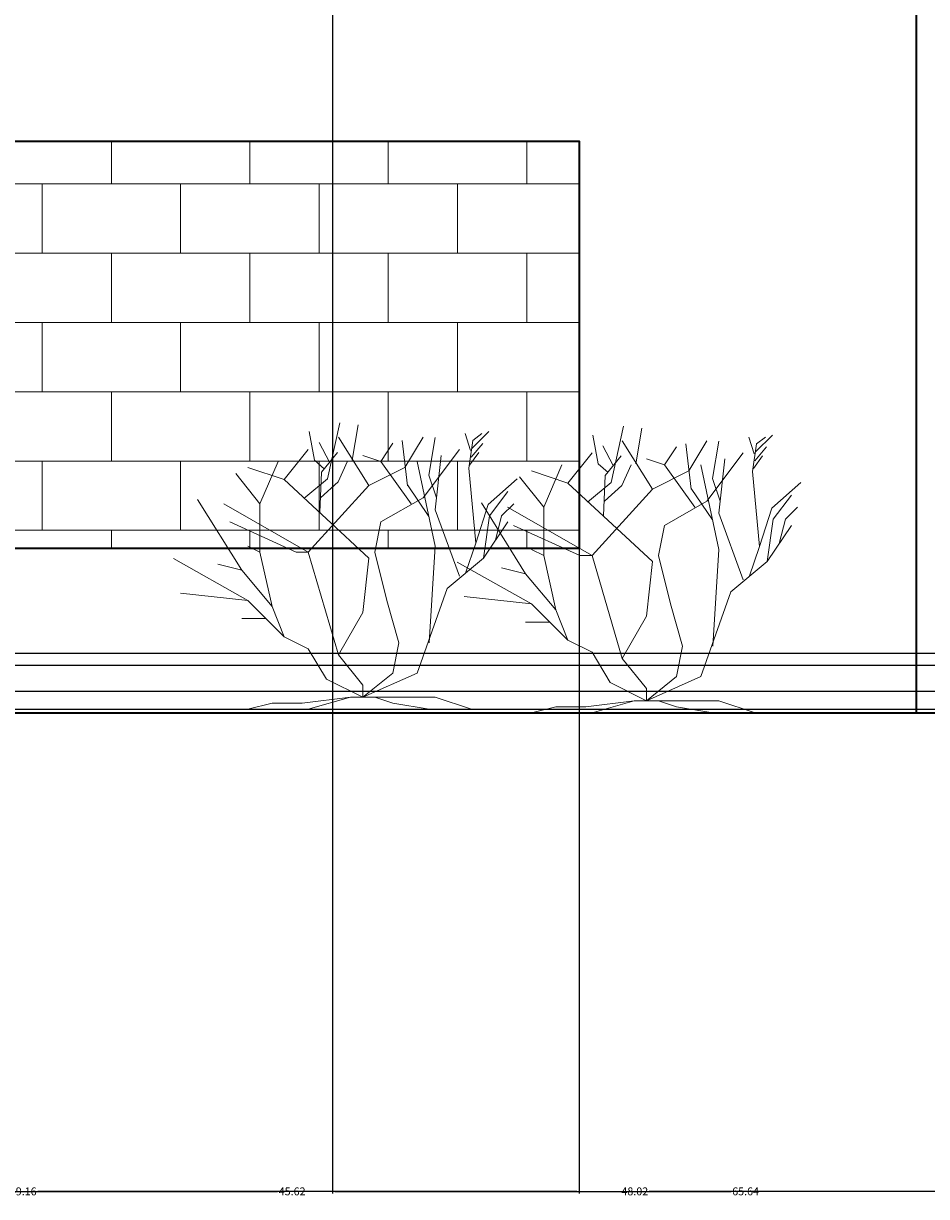
# Model space of a CAD drawing. Units: inches. Extents: x -13 to 809, y 112 to 656.
# Tile 8 of 55: x 186 to 257, y 112 to 205. Entities that reach past the tile are written whole.
import ezdxf

# ---------------------------------------------------------------- set-up
doc = ezdxf.new("R2010")
doc.units = ezdxf.units.IN
doc.header["$MEASUREMENT"] = 0
for name, color, linetype, lineweight in [('A-ANNO-DIMS', 2, 'Continuous', 18), ('A-ELEV', 7, 'Continuous', 35), ('A-ELEV-PATT', 8, 'Continuous', 13), ('L-PLNT', 3, 'Continuous', 18)]:
    doc.layers.add(name, color=color, linetype=linetype, lineweight=lineweight)
doc.styles.get("Standard").update_dxf_attribs({"font": 'arial.ttf'})
doc.dimstyles.get("Standard").update_dxf_attribs({"dimtxt": 0.625, "dimasz": 0.18, "dimexe": 0.18, "dimexo": 0.0625, "dimgap": 0.09, "dimtad": 0, "dimtih": 1, "dimtoh": 1, "dimdec": 4, "dimzin": 0, "dimdsep": 46, "dimlunit": 4, "dimtxsty": 'Standard', "dimcen": 0.09, "dimadec": 0, "dimazin": 0, "dimtfac": 1, "dimtdec": 4, "dimtofl": 0, "dimtmove": 0, "dimatfit": 3, "dimfxl": 1, "dimtolj": 1, "dimtzin": 0, "dimarcsym": 0})

# ---------------------------------------------------------------- blocks, each defined once
blk = doc.blocks.new('Shrub - elevation')
for p, q in [((-11.433, 18.289), (-10.457, 22.749)), ((-9.48, 19.775), (-8.992, 22.592)), ((-12.471, 19.775), (-12.898, 22.044)), ((-8.16, 17.76), (-10.56, 21.6)), ((-5.28, 19.2), (-3.84, 21.6)), ((-3.377, 18.602), (-2.888, 21.575)), ((-0.508, 21.888), (-0.081, 20.558)), ((0.041, 20.714), (1.384, 22.044)), ((0.102, 21.34), (0.835, 21.888)), ((-14.88, 18.24), (-12.96, 20.64)), ((-11.28, 19.619), (-12.104, 21.184)), ((-7.2, 19.68), (-6.24, 21.12)), ((-5.086, 17.741), (-5.513, 21.34)), ((-3.84, 16.8), (-0.96, 20.64)), ((-0.203, 19.149), (0.102, 21.34)), ((-0.02, 20.01), (0.896, 21.105)), ((-16.8, 16.32), (-15.36, 19.68)), ((-11.677, 19.071), (-12.471, 19.775)), ((-11.921, 18.836), (-10.64, 20.401)), ((-10.579, 18.054), (-9.846, 19.697)), ((-7.2, 19.68), (-8.64, 20.16)), ((-4.8, 16.32), (-7.2, 19.68)), ((-2.88, 12.96), (-4.32, 19.68)), ((-2.88, 15.84), (-2.4, 20.16)), ((-0.142, 19.384), (0.59, 20.401)), ((-16.8, 16.32), (-18.72, 18.72)), ((-14.88, 18.24), (-17.76, 19.2)), ((-12.043, 15.628), (-11.921, 18.836)), ((-8.16, 17.76), (-5.28, 19.2)), ((0.346, 13.203), (-0.203, 19.149)), ((-8.16, 12), (-14.88, 18.24)), ((-13.325, 16.724), (-11.433, 18.289)), ((-12.96, 12.48), (-8.16, 17.76)), ((-11.982, 16.802), (-10.579, 18.054)), ((-3.377, 15.315), (-5.086, 17.819)), ((-2.766, 16.802), (-3.377, 18.602)), ((1.323, 16.254), (3.642, 18.289)), ((-7.2, 14.88), (-3.84, 16.8)), ((1.44, 15.36), (2.88, 17.28)), ((-18.24, 11.04), (-21.755, 16.655)), ((-12.96, 12.48), (-19.68, 16.32)), ((-16.8, 12.48), (-16.8, 16.32)), ((-0.96, 10.56), (-2.88, 15.84)), ((0.346, 13.203), (1.323, 16.254)), ((2.4, 15.36), (3.36, 16.32)), ((0.96, 12), (1.44, 15.36)), ((1.92, 13.44), (2.4, 15.36)), ((-13.92, 12.48), (-19.2, 14.88)), ((-7.68, 12.48), (-7.2, 14.88)), ((0.96, 12), (2.88, 14.88)), ((-0.48, 10.8), (0.346, 13.203)), ((-16.8, 12.48), (-17.76, 12.96)), ((-15.84, 8.16), (-16.8, 12.48)), ((-12.96, 12.48), (-13.92, 12.48)), ((-10.56, 4.32), (-12.96, 12.48)), ((-6.72, 8.64), (-7.68, 12.48)), ((-3.36, 5.28), (-2.88, 12.96)), ((-17.76, 8.64), (-23.663, 11.961)), ((-18.24, 11.04), (-20.16, 11.52)), ((-8.64, 7.68), (-8.16, 12)), ((-1.92, 9.6), (0.96, 12)), ((-15.84, 8.16), (-18.24, 11.04)), ((-4.32, 2.88), (-1.92, 9.6)), ((-17.76, 8.64), (-23.128, 9.222)), ((-14.88, 5.76), (-17.76, 8.64)), ((-5.76, 5.28), (-6.72, 8.64)), ((-14.88, 5.76), (-15.84, 8.16)), ((-10.56, 4.32), (-8.64, 7.68)), ((-16.32, 7.2), (-18.24, 7.2)), ((-12.96, 4.8), (-14.88, 5.76)), ((-11.52, 2.4), (-12.96, 4.8)), ((-6.24, 2.88), (-5.76, 5.28)), ((-8.64, 1.92), (-10.56, 4.32)), ((-8.64, 0.96), (-4.32, 2.88)), ((-8.64, 0.96), (-6.24, 2.88)), ((-8.64, 0.96), (-11.52, 2.4)), ((-8.64, 0.96), (-8.64, 1.92)), ((-9.6, 0.96), (-13.44, 0.48)), ((-9.6, 0.96), (-12.96, 0)), ((-9.6, 0.96), (-7.68, 0.96)), ((-8.64, 0.96), (-2.88, 0.96)), ((-7.68, 0.96), (-6.24, 0.48)), ((-2.88, 0.96), (0, 0)), ((-15.84, 0.48), (-17.76, 0)), ((-13.44, 0.48), (-15.84, 0.48)), ((-6.24, 0.48), (-3.36, 0))]:
    blk.add_line(p, q)
blk = doc.blocks.new('*D14')
at = {"layer": 'A-ANNO-DIMS', "color": 0, "lineweight": -2, "transparency": 16777216}
for p, q in [((210.079, 223.038), (210.079, 112.34)), ((160.918, 210.457), (160.918, 112.34)), ((161.098, 112.52), (184.342, 112.52)), ((209.899, 112.52), (186.656, 112.52))]:
    blk.add_line(p, q, dxfattribs=at)
at = {"layer": 'A-ANNO-DIMS', "color": 0, "transparency": 16777216}
for points in [[(161.098, 112.55), (161.098, 112.49), (160.918, 112.52)], [(209.899, 112.55), (209.899, 112.49), (210.079, 112.52)]]:
    blk.add_solid(points, dxfattribs=at)
at = {"layer": 'Defpoints', "color": 0, "transparency": 16777216}
for p in [(210.079, 223.1), (160.918, 210.52), (210.079, 112.52)]:
    blk.add_point(p, dxfattribs=at)
at = {"layer": 'A-ANNO-DIMS', "color": 0, "transparency": 16777216, "insert": (185.499, 112.52), "char_height": 0.625, "attachment_point": 5}
blk.add_mtext('\\A1;49.16', dxfattribs=at)
blk = doc.blocks.new('*D15')
at = {"layer": 'A-ANNO-DIMS', "color": 0, "lineweight": -2, "transparency": 16777216}
for p, q in [((210.079, 223.038), (210.079, 112.34)), ((258.102, 210.722), (258.102, 112.34)), ((210.259, 112.52), (232.937, 112.52)), ((257.922, 112.52), (235.245, 112.52))]:
    blk.add_line(p, q, dxfattribs=at)
at = {"layer": 'A-ANNO-DIMS', "color": 0, "transparency": 16777216}
for points in [[(210.259, 112.55), (210.259, 112.49), (210.079, 112.52)], [(257.922, 112.55), (257.922, 112.49), (258.102, 112.52)]]:
    blk.add_solid(points, dxfattribs=at)
at = {"layer": 'Defpoints', "color": 0, "transparency": 16777216}
for p in [(210.079, 223.1), (258.102, 210.785), (258.102, 112.52)]:
    blk.add_point(p, dxfattribs=at)
at = {"layer": 'A-ANNO-DIMS', "color": 0, "transparency": 16777216, "insert": (234.091, 112.52), "char_height": 0.625, "attachment_point": 5}
blk.add_mtext('\\A1;48.02', dxfattribs=at)
blk = doc.blocks.new('*D89')
at = {"layer": 'A-ANNO-DIMS', "color": 0, "lineweight": -2, "transparency": 16777216}
for p, q in [((184.056, 195.828), (184.056, 112.34)), ((229.674, 195.828), (229.674, 112.34)), ((184.236, 112.52), (205.711, 112.52)), ((229.494, 112.52), (208.019, 112.52))]:
    blk.add_line(p, q, dxfattribs=at)
at = {"layer": 'A-ANNO-DIMS', "color": 0, "transparency": 16777216}
for points in [[(184.236, 112.55), (184.236, 112.49), (184.056, 112.52)], [(229.494, 112.55), (229.494, 112.49), (229.674, 112.52)]]:
    blk.add_solid(points, dxfattribs=at)
at = {"layer": 'Defpoints', "color": 0, "transparency": 16777216}
for p in [(184.056, 195.891), (229.674, 195.891), (229.674, 112.52)]:
    blk.add_point(p, dxfattribs=at)
at = {"layer": 'A-ANNO-DIMS', "color": 0, "transparency": 16777216, "insert": (206.865, 112.52), "char_height": 0.625, "attachment_point": 5}
blk.add_mtext('\\A1;45.62', dxfattribs=at)
blk = doc.blocks.new('*D111')
at = {"layer": 'A-ANNO-DIMS', "color": 0, "lineweight": -2, "transparency": 16777216}
for p, q in [((210.079, 361.229), (210.079, 112.34)), ((160.918, 324.457), (160.918, 112.34)), ((161.098, 112.52), (184.342, 112.52)), ((209.899, 112.52), (186.656, 112.52))]:
    blk.add_line(p, q, dxfattribs=at)
at = {"layer": 'A-ANNO-DIMS', "color": 0, "transparency": 16777216}
for points in [[(161.098, 112.55), (161.098, 112.49), (160.918, 112.52)], [(209.899, 112.55), (209.899, 112.49), (210.079, 112.52)]]:
    blk.add_solid(points, dxfattribs=at)
at = {"layer": 'Defpoints', "color": 0, "transparency": 16777216}
for p in [(210.079, 361.292), (160.918, 324.52), (210.079, 112.52)]:
    blk.add_point(p, dxfattribs=at)
at = {"layer": 'A-ANNO-DIMS', "color": 0, "transparency": 16777216, "insert": (185.499, 112.52), "char_height": 0.625, "attachment_point": 5}
blk.add_mtext('\\A1;49.16', dxfattribs=at)
blk = doc.blocks.new('*D112')
at = {"layer": 'A-ANNO-DIMS', "color": 0, "lineweight": -2, "transparency": 16777216}
for p, q in [((210.079, 361.229), (210.079, 112.34)), ((275.715, 361.229), (275.715, 112.34)), ((210.259, 112.52), (241.752, 112.52)), ((275.535, 112.52), (244.042, 112.52))]:
    blk.add_line(p, q, dxfattribs=at)
at = {"layer": 'A-ANNO-DIMS', "color": 0, "transparency": 16777216}
for points in [[(210.259, 112.55), (210.259, 112.49), (210.079, 112.52)], [(275.535, 112.55), (275.535, 112.49), (275.715, 112.52)]]:
    blk.add_solid(points, dxfattribs=at)
at = {"layer": 'Defpoints', "color": 0, "transparency": 16777216}
for p in [(210.079, 361.292), (275.715, 361.292), (275.715, 112.52)]:
    blk.add_point(p, dxfattribs=at)
at = {"layer": 'A-ANNO-DIMS', "color": 0, "transparency": 16777216, "insert": (242.897, 112.52), "char_height": 0.625, "attachment_point": 5}
blk.add_mtext('\\A1;65.64', dxfattribs=at)
blk = doc.blocks.new('*D115')
at = {"layer": 'A-ANNO-DIMS', "color": 0, "lineweight": -2, "transparency": 16777216}
for p, q in [((311.4, 210.785), (-12.099, 210.785)), ((-11.919, 210.605), (-11.919, 181.062)), ((-11.919, 150.7), (-11.919, 180.243)), ((311.637, 150.52), (-12.099, 150.52))]:
    blk.add_line(p, q, dxfattribs=at)
at = {"layer": 'A-ANNO-DIMS', "color": 0, "transparency": 16777216}
for points in [[(-11.949, 210.605), (-11.889, 210.605), (-11.919, 210.785)], [(-11.949, 150.7), (-11.889, 150.7), (-11.919, 150.52)]]:
    blk.add_solid(points, dxfattribs=at)
at = {"layer": 'Defpoints', "color": 0, "transparency": 16777216}
for p in [(-11.919, 210.785), (311.463, 210.785), (311.699, 150.52)]:
    blk.add_point(p, dxfattribs=at)
at = {"layer": 'A-ANNO-DIMS', "color": 0, "transparency": 16777216, "insert": (-11.919, 180.652), "char_height": 0.625, "attachment_point": 5}
blk.add_mtext('\\A1;60.27', dxfattribs=at)
blk = doc.blocks.new('*D117')
at = {"layer": 'A-ANNO-DIMS', "color": 0, "lineweight": -2, "transparency": 16777216}
for p, q in [((260.642, 154.272), (-12.099, 154.272)), ((-11.919, 154.092), (-11.919, 152.938)), ((-11.919, 150.965), (-11.919, 152.119)), ((258.04, 150.785), (-12.099, 150.785))]:
    blk.add_line(p, q, dxfattribs=at)
at = {"layer": 'A-ANNO-DIMS', "color": 0, "transparency": 16777216}
for points in [[(-11.949, 154.092), (-11.889, 154.092), (-11.919, 154.272)], [(-11.949, 150.965), (-11.889, 150.965), (-11.919, 150.785)]]:
    blk.add_solid(points, dxfattribs=at)
at = {"layer": 'Defpoints', "color": 0, "transparency": 16777216}
for p in [(260.705, 154.272), (-11.919, 150.785), (258.102, 150.785)]:
    blk.add_point(p, dxfattribs=at)
at = {"layer": 'A-ANNO-DIMS', "color": 0, "transparency": 16777216, "insert": (-11.919, 152.529), "char_height": 0.625, "attachment_point": 5}
blk.add_mtext('\\A1;3.487', dxfattribs=at)
blk = doc.blocks.new('*D131')
at = {"layer": 'A-ANNO-DIMS', "color": 0, "lineweight": -2, "transparency": 16777216}
for p, q in [((368.876, 155.214), (-12.099, 155.214)), ((-11.919, 155.034), (-11.919, 154.123)), ((-11.919, 152.394), (-11.919, 153.305)), ((365.876, 152.214), (-12.099, 152.214))]:
    blk.add_line(p, q, dxfattribs=at)
at = {"layer": 'A-ANNO-DIMS', "color": 0, "transparency": 16777216}
for points in [[(-11.949, 155.034), (-11.889, 155.034), (-11.919, 155.214)], [(-11.949, 152.394), (-11.889, 152.394), (-11.919, 152.214)]]:
    blk.add_solid(points, dxfattribs=at)
at = {"layer": 'Defpoints', "color": 0, "transparency": 16777216}
for p in [(368.938, 155.214), (-11.919, 152.214), (365.938, 152.214)]:
    blk.add_point(p, dxfattribs=at)
at = {"layer": 'A-ANNO-DIMS', "color": 0, "transparency": 16777216, "insert": (-11.919, 153.714), "char_height": 0.625, "attachment_point": 5}
blk.add_mtext('\\A1;3.00', dxfattribs=at)

msp = doc.modelspace()

# ---------------------------------------------------------------- hatches: boundary and pattern name
at = {"layer": 'A-ELEV-PATT'}
h = msp.add_hatch(dxfattribs=at)
h.set_pattern_fill('BRICK', color=256, scale=22)
h.paths.add_polyline_path([(113.3574, 195.8907), (76.4733, 195.8907), (76.4733, 163.5637), (113.3574, 163.5637)])
h.paths.add_polyline_path([(167.4098, 195.8907), (129.2551, 195.8907), (129.2551, 163.5637), (167.4098, 163.5637)])
h.paths.add_polyline_path([(229.6736, 195.8907), (184.0557, 195.8907), (184.0557, 163.5637), (229.6736, 163.5637)])

# ---------------------------------------------------------------- linework, layer by layer
at = {"layer": 'A-ELEV'}
for p, q in [((256.4464, 210.5199), (256.4464, 150.5199)), ((109.5888, 150.5199), (649.5888, 150.5199))]:
    msp.add_line(p, q, dxfattribs=at)
msp.add_lwpolyline([(76.4733, 195.8907), (229.6736, 195.8907), (229.6736, 163.5637), (76.4733, 163.5637)], close=True, dxfattribs=at)

# ---------------------------------------------------------------- block references
at = {"layer": 'L-PLNT'}
for p in [(221.1108, 150.7954), (243.6539, 150.5199)]:
    msp.add_blockref('Shrub - elevation', p, dxfattribs=at)

# ---------------------------------------------------------------- dimensions: what is measured, and where the dimension line sits
at = {"layer": 'A-ANNO-DIMS'}
for base, p1, p2, picture, middle in [((210.0791, 112.5199), (160.9184, 324.5199), (210.0791, 361.2915), '*D111', (185.4988, 112.5199)), ((275.7145, 112.5199), (210.0791, 361.2915), (275.7145, 361.2915), '*D112', (242.8968, 112.5199)), ((210.0791, 112.5199), (160.9184, 210.5199), (210.0791, 223.1), '*D14', (185.4988, 112.5199)), ((258.1022, 112.5199), (210.0791, 223.1), (258.1022, 210.7849), '*D15', (234.0906, 112.5199)), ((229.6736, 112.5199), (184.0557, 195.8907), (229.6736, 195.8907), '*D89', (206.8646, 112.5199))]:
    dim = msp.add_linear_dim(base=base, p1=p1, p2=p2, dimstyle='Standard', override={"dimdec": 2, "dimlfac": 1, "dimrnd": 0, "dimzin": 0, "dimdsep": 46, "dimlunit": 2}, dxfattribs=at)
    dim.commit()
    dim.dimension.update_dxf_attribs({"geometry": picture, "text_midpoint": middle})
for base, p1, p2, override, picture, middle in [((-11.91915, 210.78493), (311.6991, 150.51989), (311.46269, 210.78493), {"dimdec": 2, "dimlfac": 1, "dimrnd": 0, "dimzin": 0, "dimdsep": 46, "dimlunit": 2}, '*D115', (-11.91915, 180.65241)), ((-11.9191, 152.2141), (368.9383, 155.2141), (365.9383, 152.2141), {"dimdec": 2, "dimlfac": 1, "dimrnd": 0, "dimzin": 0, "dimdsep": 46, "dimlunit": 2}, '*D131', (-11.9191, 153.7141)), ((-11.9191, 150.7849), (260.7048, 154.2723), (258.1022, 150.7849), {"dimdec": 3, "dimlfac": 1, "dimrnd": 0, "dimzin": 0, "dimdsep": 46, "dimlunit": 2}, '*D117', (-11.9191, 152.5286))]:
    dim = msp.add_linear_dim(base=base, p1=p1, p2=p2, angle=90, dimstyle='Standard', override=override, dxfattribs=at)
    dim.commit()
    dim.dimension.update_dxf_attribs({"geometry": picture, "text_midpoint": middle})

doc.saveas('drawing.dxf')
